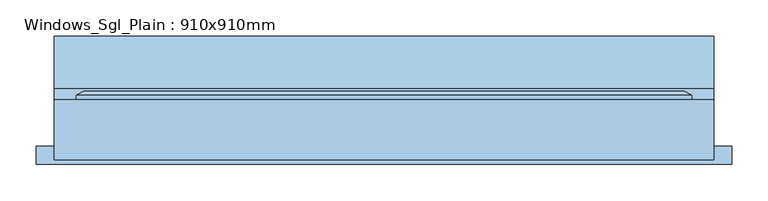
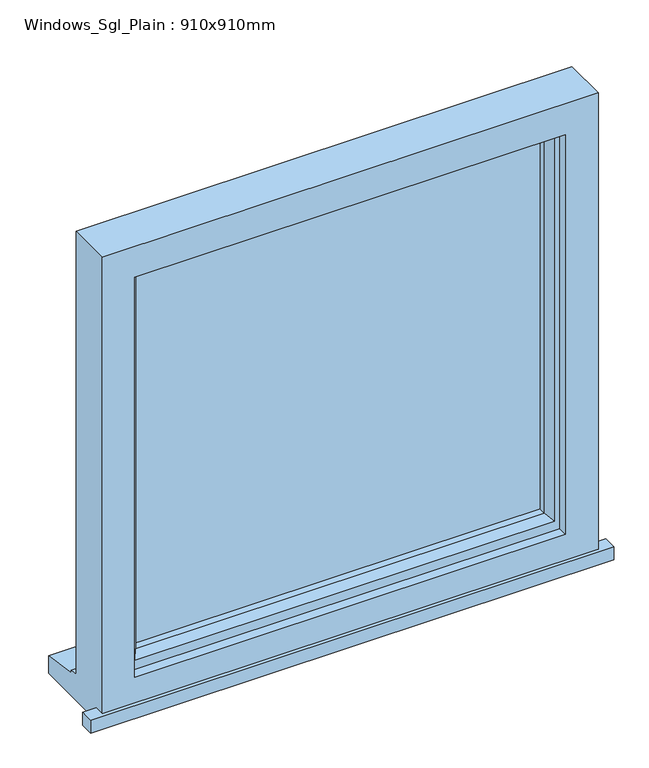
"""IFC4 building model written with IfcOpenShell, lengths in millimetres: window geometry, Windows_Sgl_Plain : 910x910mm."""

from ifc_helpers import new_model, si_unit, frame, origin, place, context, project, spatial, polyline, outline, extrude, faceted_brep, source, transform, mapped, element, save


def windows_sgl_plain_910x910mm_53772929(model_context):
    return source(origin(), model_context, "Body", "SolidModel", [
        extrude(outline(polyline([(-480.0, -73.6934322), (-480.0, -48.6934322), (-455.0, -48.6934322), (-455.0, -67.3934322), (455.0, -67.3934322), (455.0, -48.6934322), (480.0, -48.6934322), (480.0, -73.6934322), (-480.0, -73.6934322)])), frame((0.0, 0.0, 1200.0), z_axis=(0.0, 0.0, 1.0), x_axis=(1.0, 0.0, 0.0)), (0.0, 0.0, 1.0), 25.0),
        faceted_brep([(-455.0, -67.3934322, 1200.0), (455.0, -67.3934322, 1200.0), (455.0, -67.3934322, 2110.0), (-455.0, -67.3934322, 2110.0), (-395.0, -67.3934322, 2050.0), (395.0, -67.3934322, 2050.0), (395.0, -67.3934322, 1275.0), (-395.0, -67.3934322, 1275.0), (-455.0, 15.6065678, 2110.0), (-455.0, 15.6065678, 1251.0), (-455.0, 30.6065678, 1249.68767), (-455.0, 30.6065678, 1244.7449676), (-455.0, 103.1065678, 1233.8088847), (-455.0, 103.1065678, 1200.0), (455.0, 15.6065678, 2110.0), (455.0, 15.6065678, 1251.0), (-415.0, 15.6065678, 2070.0), (-415.0, 15.6065678, 1263.0), (415.0, 15.6065678, 1263.0), (415.0, 15.6065678, 2070.0), (-415.0, -49.3934322, 2070.0), (-415.0, -49.3934322, 1263.0), (415.0, -49.3934322, 2070.0), (415.0, -49.3934322, 1263.0), (-395.0, -49.3934322, 2050.0), (-395.0, -49.3934322, 1275.0), (395.0, -49.3934322, 1275.0), (395.0, -49.3934322, 2050.0), (455.0, 103.1065678, 1200.0), (455.0, 103.1065678, 1233.8088847), (455.0, 30.6065678, 1244.7449676), (455.0, 30.6065678, 1249.68767)], [[[0, 1, 2, 3], [4, 5, 6, 7]], [[0, 3, 8, 9, 10, 11, 12, 13]], [[9, 8, 14, 15], [16, 17, 18, 19]], [[17, 16, 20, 21]], [[20, 22, 23, 21], [24, 25, 26, 27]], [[24, 4, 7, 25]], [[3, 2, 14, 8]], [[16, 19, 22, 20]], [[5, 4, 24, 27]], [[15, 14, 2, 1, 28, 29, 30, 31]], [[19, 18, 23, 22]], [[5, 27, 26, 6]], [[28, 1, 0, 13]], [[29, 28, 13, 12]], [[30, 29, 12, 11]], [[31, 30, 11, 10]], [[15, 31, 10, 9]], [[21, 23, 18, 17]], [[7, 6, 26, 25]]]),
        extrude(outline(polyline([(385.0, -20.3934322), (-385.0, -20.3934322), (-385.0, 3.6065678), (385.0, 3.6065678), (385.0, -20.3934322)])), frame((0.0, 0.0, 1293.0), z_axis=(0.0, 0.0, 1.0), x_axis=(1.0, 0.0, 0.0)), (0.0, 0.0, 1.0), 747.0),
        faceted_brep([(-425.0, 15.6065678, 2080.0), (-425.0, 21.3800705, 2080.0), (-425.0, 21.3800705, 1253.0), (-425.0, 15.6065678, 1253.0), (-415.0, -49.3934322, 2070.0), (-415.0, 15.6065678, 2070.0), (-415.0, 15.6065678, 1263.0), (-415.0, -49.3934322, 1263.0), (-375.0, -34.9005323, 2030.0), (-385.1480377, -49.3934322, 2040.1480377), (-385.1480377, -49.3934322, 1292.8519623), (-375.0, -34.9005323, 1303.0), (-375.0, -20.3934322, 2030.0), (-375.0, -20.3934322, 1303.0), (-385.0, 3.6065678, 2040.0), (-385.0, -20.3934322, 2040.0), (-385.0, -20.3934322, 1293.0), (-385.0, 3.6065678, 1293.0), (-375.0, 21.3800705, 2030.0), (-375.0, 3.6065678, 2030.0), (-375.0, 3.6065678, 1303.0), (-375.0, 21.3800705, 1303.0), (-392.4457548, 27.1535732, 2047.4457548), (-392.4457548, 27.1535732, 1285.5542452), (-414.2153903, 27.1535732, 2069.2153903), (-414.2153903, 27.1535732, 1263.7846097), (425.0, 21.3800705, 1253.0), (425.0, 15.6065678, 1253.0), (415.0, 15.6065678, 1263.0), (415.0, -49.3934322, 1263.0), (385.1480377, -49.3934322, 1292.8519623), (375.0, -34.9005323, 1303.0), (375.0, -20.3934322, 1303.0), (385.0, -20.3934322, 1293.0), (385.0, 3.6065678, 1293.0), (375.0, 3.6065678, 1303.0), (375.0, 21.3800705, 1303.0), (392.4457548, 27.1535732, 1285.5542452), (414.2153903, 27.1535732, 1263.7846097), (425.0, 21.3800705, 2080.0), (425.0, 15.6065678, 2080.0), (415.0, 15.6065678, 2070.0), (415.0, -49.3934322, 2070.0), (385.1480377, -49.3934322, 2040.1480377), (375.0, -34.9005323, 2030.0), (375.0, -20.3934322, 2030.0), (385.0, -20.3934322, 2040.0), (385.0, 3.6065678, 2040.0), (375.0, 3.6065678, 2030.0), (375.0, 21.3800705, 2030.0), (392.4457548, 27.1535732, 2047.4457548), (414.2153903, 27.1535732, 2069.2153903)], [[[0, 1, 2, 3]], [[4, 5, 6, 7]], [[8, 9, 10, 11]], [[12, 8, 11, 13]], [[14, 15, 16, 17]], [[18, 19, 20, 21]], [[22, 18, 21, 23]], [[1, 24, 25, 2]], [[3, 2, 26, 27]], [[7, 6, 28, 29]], [[11, 10, 30, 31]], [[13, 11, 31, 32]], [[17, 16, 33, 34]], [[21, 20, 35, 36]], [[23, 21, 36, 37]], [[2, 25, 38, 26]], [[27, 26, 39, 40]], [[29, 28, 41, 42]], [[31, 30, 43, 44]], [[32, 31, 44, 45]], [[34, 33, 46, 47]], [[36, 35, 48, 49]], [[37, 36, 49, 50]], [[26, 38, 51, 39]], [[40, 39, 1, 0]], [[3, 27, 40, 0], [5, 41, 28, 6]], [[42, 41, 5, 4]], [[7, 29, 42, 4], [9, 43, 30, 10]], [[44, 43, 9, 8]], [[45, 44, 8, 12]], [[15, 46, 33, 16], [13, 32, 45, 12]], [[47, 46, 15, 14]], [[17, 34, 47, 14], [19, 48, 35, 20]], [[49, 48, 19, 18]], [[50, 49, 18, 22]], [[24, 51, 38, 25], [23, 37, 50, 22]], [[39, 51, 24, 1]]]),
    ])


if __name__ == "__main__":
    model = new_model("IFC4")
    model_context = context("Model", 3, world=origin())
    ifc_project = project(units=[si_unit("LENGTHUNIT", "METRE", prefix="MILLI")], contexts=[model_context])
    site = spatial("IfcSite", under=ifc_project)
    building = spatial("IfcBuilding", under=site)
    placement = place(None, origin())
    windows_sgl_plain_910x910mm_shape = windows_sgl_plain_910x910mm_53772929(model_context)
    element("IfcWindow", 1, ObjectType="Windows_Sgl_Plain : 910x910mm", at=placement, inside=building, context=model_context, shape_type="MappedRepresentation", body=[
        mapped(windows_sgl_plain_910x910mm_shape, transform((0.0, 0.0, 0.0), x_axis=(1.0, 0.0, 0.0), y_axis=(0.0, 1.0, 0.0), z_axis=(0.0, 0.0, 1.0))),
    ])
    save(model, "model.ifc")

# Revit data of these elements
# Type "Windows_Sgl_Plain : 910x910mm"
#   Type Mark = "44"
#   Operation = "SinglePanel"
#   Construction Type Id = "SGL"
#   Manufacturer = "Revit"
#   Keynote = "L10"
#   Analytic Construction = "Large single-glazed windows"
#   Wrap Layers (Ext) from Ext = 0' - 4.03543"
#   Wrap Layers (Int) from Ext = 0' - 6.98819"
#   Window Board Projection = 0' - 0.98425"
#   Window Board Extension = 0' - 0.98425"
#   Visual Light Transmittance = 0.9
#   Solar Heat Gain Coefficient = 0.86
#   Rough Width = 2' - 11.82677"
#   Rough Height = 2' - 11.82677"
#   Height = 2' - 11.82677"
#   Width = 2' - 11.82677"
#   Heat Transfer Coefficient (U) = 5.5617 W/(m²·K)
#   Glazing Thickness = 0' - 0.94488"
#   FrameOffset - External = 0' - 1.9685"
#   Frame Depth = 0' - 2.55906"
#   Default Head Height = 6' - 11.07087"
#   Cill Depth = 0' - 3.44488"
#   Cavity Closer Width = 0' - 1.9685"
#   Cavity Closer Offset from Ext = 0' - 4.03543"
#   Cavity Closer Depth = 0' - 3.34646"
#   Define Thermal Properties by = 1
#   Vis - Cavity Closers = yes
#   Define Thermal Properties by = 1
#   Material Trim = Window Frame
#   Material Glass = Glass
#   Material Frame = Window Frame
#   Wall Closure = (empty or 0)
# Element 1 (IfcWindow, "Windows_Sgl_Plain : 910x910mm")
#   Materials on its faces: "Window Frame", "Glass"
# Materials
#   "Window Frame": colour RGB 249 249 249, transparency 0, Keynote = "L10", Cost = 0
#   "Glass": class "Glass", colour RGB 0 128 192, transparency 0.9, Description = "Soda Lime Glass", Cost = 0
